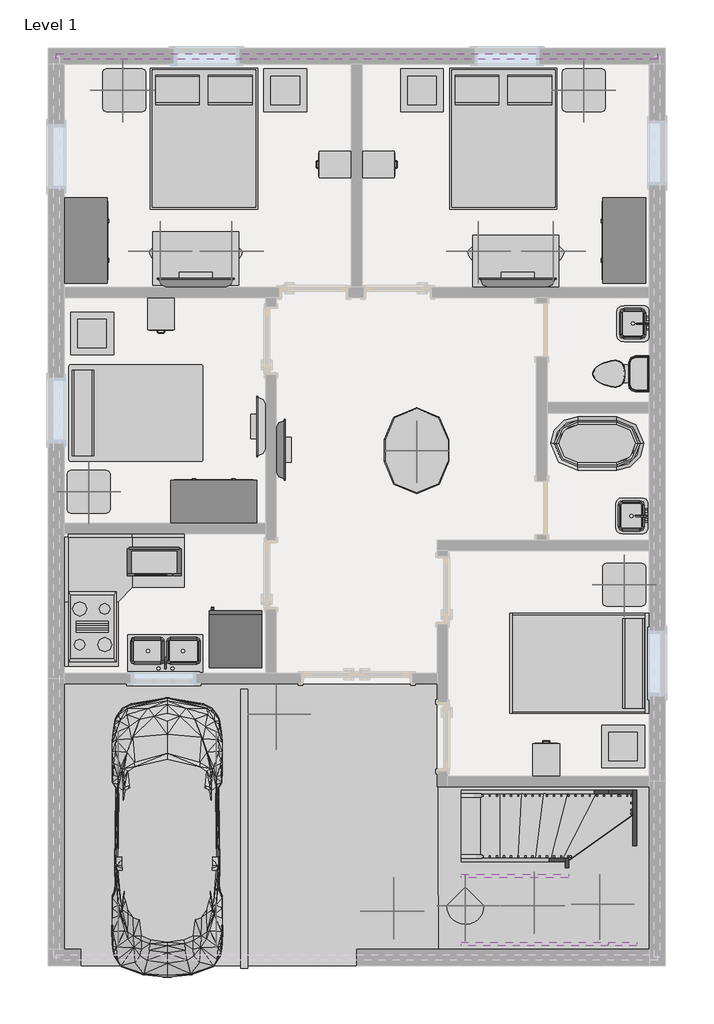
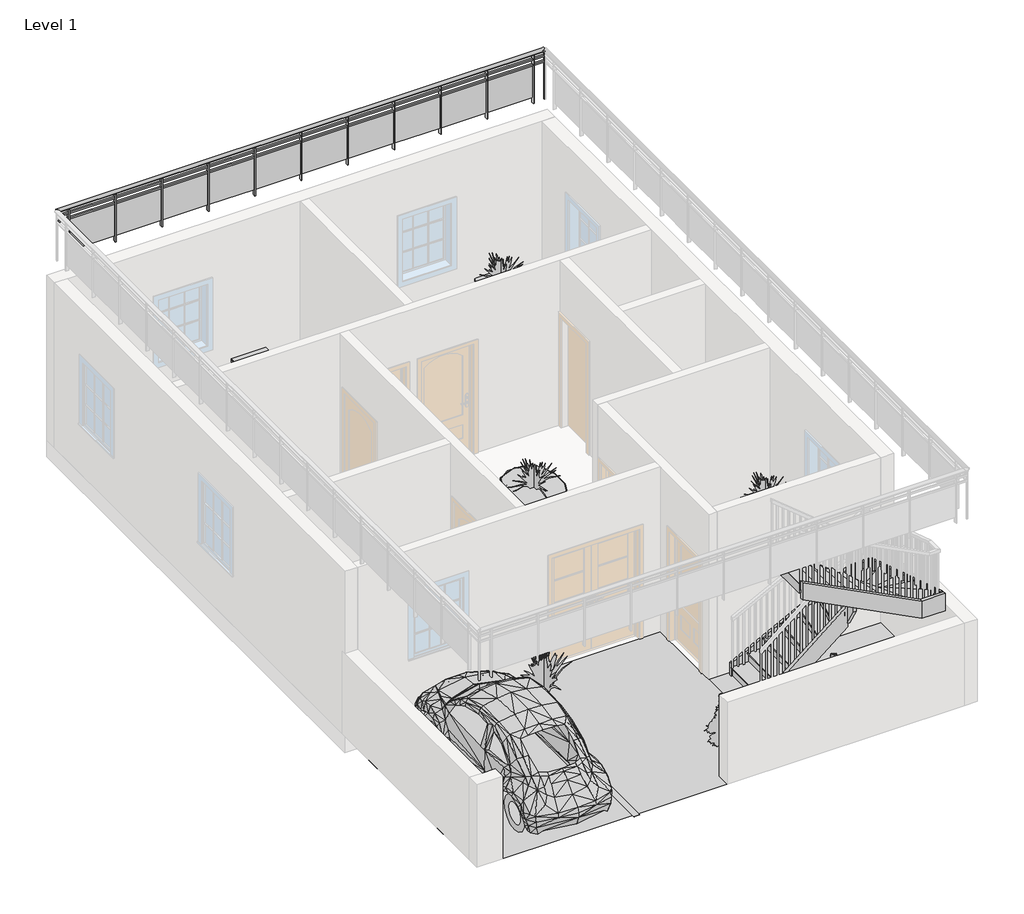
# One storey, part 4 of 4: 27 furniture elements, 14 geographic elements, 8 members, 7 flow terminals, 7 proxies, 1 railing, 1 stair flight.
"""IFC4 building model written with IfcOpenShell, lengths in millimetres."""

from ifc_helpers import new_model, si_unit, point, frame, origin, place, context, project, spatial, polyline, ellipse_curve, trimmed, outline, extrude, triangles, transform, mapped, element, save
from ifc_brep_helpers import plane_surface, extruded_surface, advanced_brep
from components import proxy_bb1e6e30, proxy_8a8d5ab2, parking_space_9_x_18_90_deg_c935943f, rpc_beetle_rpc_beetle_3ce7ba48, proxy_a13a33b2, flow_terminal_accce45a, flow_terminal_a53be723, flow_terminal_62a433f7, toilet_domestic_3d_toilet_domestic_3d_f7549cf7, toilet_domestic_3d_toilet_domestic_3d_183bbd19, flow_terminal_159a3241, furniture_1d2926bd, furniture_096e7f55, furniture_0253826f, furniture_bb55ed6b, furniture_9fa109b2, furniture_56245f3a, furniture_7a3aaa4f, furniture_b5c51a22, furniture_be1c6672, furniture_31d08a24, furniture_1bba2e14, furniture_005e41fd, rpc_plant_tropical_55f6ff97, rpc_plant_tropical_agave_1_5_93a2a214, rpc_plant_tropical_jungle_flame_3_9c4808c2, stair_flight_2bffc1af

model = new_model("IFC4")

# Units and contexts
model_context = context("Model", 3, world=origin())
ifc_project = project(units=[si_unit("LENGTHUNIT", "METRE", prefix="MILLI")], contexts=[model_context])

# Site, building, storey
site = spatial("IfcSite", under=ifc_project)
building = spatial("IfcBuilding", under=site)
storey = spatial("IfcBuildingStorey", under=building, Name="Level 1", Elevation=0.0)

# Proxies
placement = place(None, origin())
element("IfcBuildingElementProxy", 1, Name="Building Element Proxy", at=placement, inside=storey, context=model_context, shape_type="Tessellation", body=[
    triangles([(-12848.2506409, 4171.8645401, 0.0), (-7323.7506409, 4171.8645401, 0.0), (-7307.7033646, 171.3645946, 0.0), (-12848.2506409, 171.3645946, 0.0)], [[1, 4, 2], [3, 2, 4]], closed=False),
])
element("IfcBuildingElementProxy", 2, Name="Building Element Proxy", at=placement, inside=storey, context=model_context, shape_type="Tessellation", body=[
    triangles([(-7250.1225769, 171.3645946, 0.0), (-4085.2506409, 171.3645946, 0.0), (-4085.2506409, 2711.3647339, 0.0), (-7323.7506409, 2711.3647339, 0.0), (-7329.7188812, 171.3645946, 0.0)], [[4, 5, 1], [1, 2, 3], [1, 3, 4]], closed=False),
])
proxy_shape = proxy_bb1e6e30(model_context)
element("IfcBuildingElementProxy", 3, Name="Cook Top-4 Unit : 36\" x 20\"", ObjectType="Cook Top-4 Unit : 36\" x 20\"", at=placement, inside=storey, context=model_context, shape_type="MappedRepresentation", body=[
    mapped(proxy_shape, transform((-12225.9505662, 4984.6645941, 0.0), x_axis=(0.0, 1.0, 0.0), y_axis=(-1.0, 0.0, 0.0), z_axis=(0.0, 0.0, 1.0))),
])
proxy_2_shape = proxy_8a8d5ab2(model_context)
element("IfcBuildingElementProxy", 4, Name="Microwave : 30\" x 16\" x 18\"", ObjectType="Microwave : 30\" x 16\" x 18\"", at=placement, inside=storey, context=model_context, shape_type="MappedRepresentation", body=[
    mapped(proxy_2_shape, transform((-11843.5934435, 6264.8451, 0.0), x_axis=(1.0000000000000002, 0.0, 0.0), y_axis=(0.0, 1.0000000000000002, 0.0), z_axis=(0.0, 0.0, 1.0))),
])
parking_space_9_x_18_90_deg_shape = parking_space_9_x_18_90_deg_c935943f(model_context)
element("IfcBuildingElementProxy", 5, Name="Parking Space : 9' x 18' - 90 deg", ObjectType="Parking Space : 9' x 18' - 90 deg", at=placement, inside=storey, context=model_context, shape_type="MappedRepresentation", body=[
    mapped(parking_space_9_x_18_90_deg_shape, transform((-10066.9505662, 133.2645941, 0.0), x_axis=(-1.0000000000000004, 0.0, 0.0), y_axis=(0.0, -1.0000000000000004, 0.0), z_axis=(0.0, 0.0, 1.0))),
])
rpc_beetle_rpc_beetle_shape = rpc_beetle_rpc_beetle_3ce7ba48(model_context)
element("IfcBuildingElementProxy", 6, Name="RPC Beetle : RPC Beetle", ObjectType="RPC Beetle : RPC Beetle", at=placement, inside=storey, context=model_context, shape_type="MappedRepresentation", body=[
    mapped(rpc_beetle_rpc_beetle_shape, transform((-11159.1505662, 755.5645941, 0.0), x_axis=(1.0, 0.0, 0.0), y_axis=(0.0, 1.0, 0.0), z_axis=(0.0, 0.0, 1.0))),
])
proxy_3_shape = proxy_a13a33b2(model_context)
element("IfcBuildingElementProxy", 7, Name="Refrigerator : 30\" x 32\" RH", ObjectType="Refrigerator : 30\" x 32\" RH", at=placement, inside=storey, context=model_context, shape_type="MappedRepresentation", body=[
    mapped(proxy_3_shape, transform((-10186.0130662, 4792.9656227, 0.0), x_axis=(-1.0000000000000004, 0.0, 0.0), y_axis=(0.0, -1.0000000000000004, 0.0), z_axis=(0.0, 0.0, 1.0))),
])

# Flow terminals
flow_terminal_shape = flow_terminal_accce45a(model_context)
element("IfcFlowTerminal", 8, ObjectType="Floor Drain - Round : 5\" Strainer - 2\" Drain", at=placement, inside=storey, context=model_context, shape_type="MappedRepresentation", body=[
    mapped(flow_terminal_shape, transform((-4580.5505662, 7054.7645941, 0.0), x_axis=(1.0, 0.0, 0.0), y_axis=(0.0, 1.0, 0.0), z_axis=(0.0, 0.0, 1.0))),
])
element("IfcFlowTerminal", 9, ObjectType="Floor Drain - Round : 5\" Strainer - 2\" Drain", at=placement, inside=storey, context=model_context, shape_type="MappedRepresentation", body=[
    mapped(flow_terminal_shape, transform((-4529.7505662, 9455.0645941, 0.0), x_axis=(1.0, 0.0, 0.0), y_axis=(0.0, 1.0, 0.0), z_axis=(0.0, 0.0, 1.0))),
])
flow_terminal_2_shape = flow_terminal_a53be723(model_context)
element("IfcFlowTerminal", 10, ObjectType="Sink Kitchen-Double : 42\" x 21\"", at=placement, inside=storey, context=model_context, shape_type="MappedRepresentation", body=[
    mapped(flow_terminal_2_shape, transform((-11168.8613256, 4606.0099953, 0.0), x_axis=(-1.0000000000000004, 0.0, 0.0), y_axis=(0.0, -1.0000000000000004, 0.0), z_axis=(0.0, 0.0, 1.0))),
])
flow_terminal_3_shape = flow_terminal_62a433f7(model_context)
element("IfcFlowTerminal", 11, ObjectType="Sink Vanity-Square : 20\" x 18\"", at=placement, inside=storey, context=model_context, shape_type="MappedRepresentation", body=[
    mapped(flow_terminal_3_shape, transform((-4513.0459673, 6575.1538347, 0.0), x_axis=(0.0, -1.0000000000000004, 0.0), y_axis=(1.0000000000000004, 0.0, 0.0), z_axis=(0.0, 0.0, 1.0))),
])
element("IfcFlowTerminal", 12, ObjectType="Sink Vanity-Square : 20\" x 18\"", at=placement, inside=storey, context=model_context, shape_type="MappedRepresentation", body=[
    mapped(flow_terminal_3_shape, transform((-4493.9959673, 9305.6538347, 0.0), x_axis=(0.0, -1.0, 0.0), y_axis=(1.0, 0.0, 0.0), z_axis=(0.0, 0.0, 1.0))),
])
toilet_domestic_3d_toilet_domestic_3d_shape = toilet_domestic_3d_toilet_domestic_3d_f7549cf7(model_context)
toilet_domestic_3d_toilet_domestic_3d_2_shape = toilet_domestic_3d_toilet_domestic_3d_183bbd19(model_context)
element("IfcFlowTerminal", 13, ObjectType="Toilet-Domestic-3D : Toilet-Domestic-3D", at=placement, inside=storey, context=model_context, shape_type="MappedRepresentation", body=[
    mapped(toilet_domestic_3d_toilet_domestic_3d_shape, transform((-4808.5465935, 8578.7645941, 0.0), x_axis=(0.0, -1.0000000000000007, 0.0), y_axis=(1.0000000000000007, 0.0, 0.0), z_axis=(0.0, 0.0, 1.0))),
    mapped(toilet_domestic_3d_toilet_domestic_3d_2_shape, transform((-4808.5465935, 8578.7645941, 0.0), x_axis=(0.0, -1.0000000000000007, 0.0), y_axis=(1.0000000000000007, 0.0, 0.0), z_axis=(0.0, 0.0, 1.0))),
])
flow_terminal_4_shape = flow_terminal_159a3241(model_context)
element("IfcFlowTerminal", 14, ObjectType="Tub-Free Standing-3D : 30\" x 60\"", at=placement, inside=storey, context=model_context, shape_type="MappedRepresentation", body=[
    mapped(flow_terminal_4_shape, transform((-5050.4505662, 7588.1645941, 0.0), x_axis=(0.0, 1.0, 0.0), y_axis=(-1.0, 0.0, 0.0), z_axis=(0.0, 0.0, 1.0))),
])

# Furniture
furniture_shape = furniture_1d2926bd(model_context)
element("IfcFurniture", 15, ObjectType="Bed-Box : Queen 60\" x 79\"", at=placement, inside=storey, context=model_context, shape_type="MappedRepresentation", body=[
    mapped(furniture_shape, transform((-10977.6030252, 12153.2941023, 0.0), x_axis=(1.0000000000000004, 0.0, 0.0), y_axis=(0.0, 1.0000000000000004, 0.0), z_axis=(0.0, 0.0, 1.0))),
])
element("IfcFurniture", 16, ObjectType="Bed-Box : Queen 60\" x 79\"", at=placement, inside=storey, context=model_context, shape_type="MappedRepresentation", body=[
    mapped(furniture_shape, transform((-6723.1030252, 12153.2941023, 0.0), x_axis=(1.0, 0.0, 0.0), y_axis=(0.0, 1.0, 0.0), z_axis=(0.0, 0.0, 1.0))),
])
furniture_2_shape = furniture_096e7f55(model_context)
element("IfcFurniture", 17, ObjectType="Bed-Shaker : Double 56\" x 78\"", at=placement, inside=storey, context=model_context, shape_type="MappedRepresentation", body=[
    mapped(furniture_2_shape, transform((-4313.8505662, 4444.9145941, 0.0), x_axis=(0.0, -1.0000000000000004, 0.0), y_axis=(1.0000000000000004, 0.0, 0.0), z_axis=(0.0, 0.0, 1.0))),
])
furniture_3_shape = furniture_0253826f(model_context)
element("IfcFurniture", 18, ObjectType="Bed-Standard.0001 : Double 54\" x 75\"", at=placement, inside=storey, context=model_context, shape_type="MappedRepresentation", body=[
    mapped(furniture_3_shape, transform((-11649.2456481, 7748.4760696, 0.0), x_axis=(0.0, 1.0000000000000002, 0.0), y_axis=(-1.0000000000000002, 0.0, 0.0), z_axis=(0.0, 0.0, 1.0))),
])
furniture_4_shape = furniture_bb55ed6b(model_context)
element("IfcFurniture", 19, ObjectType="Cabinet-File 2 Drawer : 15\" x 18\"", at=placement, inside=storey, context=model_context, shape_type="MappedRepresentation", body=[
    mapped(furniture_4_shape, transform((-8629.416266, 11422.6681471, 0.0), x_axis=(0.0, -1.0000000000000004, 0.0), y_axis=(1.0000000000000004, 0.0, 0.0), z_axis=(0.0, 0.0, 1.0))),
])
element("IfcFurniture", 20, ObjectType="Cabinet-File 2 Drawer : 15\" x 18\"", at=placement, inside=storey, context=model_context, shape_type="MappedRepresentation", body=[
    mapped(furniture_4_shape, transform((-8304.0848663, 11678.4610412, 0.0), x_axis=(0.0, 1.0000000000000002, 0.0), y_axis=(-1.0000000000000002, 0.0, 0.0), z_axis=(0.0, 0.0, 1.0))),
])
element("IfcFurniture", 21, ObjectType="Cabinet-File 2 Drawer : 15\" x 18\"", at=placement, inside=storey, context=model_context, shape_type="MappedRepresentation", body=[
    mapped(furniture_4_shape, transform((-11120.1541191, 9571.7988943, 0.0), x_axis=(1.0, 0.0, 0.0), y_axis=(0.0, 1.0, 0.0), z_axis=(0.0, 0.0, 1.0))),
])
element("IfcFurniture", 22, ObjectType="Cabinet-File 2 Drawer : 15\" x 18\"", at=placement, inside=storey, context=model_context, shape_type="MappedRepresentation", body=[
    mapped(furniture_4_shape, transform((-5902.2470132, 2950.230294, 0.0), x_axis=(-1.0000000000000004, 0.0, 0.0), y_axis=(0.0, -1.0000000000000004, 0.0), z_axis=(0.0, 0.0, 1.0))),
])
furniture_5_shape = furniture_9fa109b2(model_context)
element("IfcFurniture", 23, ObjectType="Dresser : 48\" x 72\" x 24\"", at=placement, inside=storey, context=model_context, shape_type="MappedRepresentation", body=[
    mapped(furniture_5_shape, transform((-12678.0135203, 10740.257854, 0.0), x_axis=(0.0, 1.0000000000000002, 0.0), y_axis=(-1.0000000000000002, 0.0, 0.0), z_axis=(0.0, 0.0, 1.0))),
])
element("IfcFurniture", 24, ObjectType="Dresser : 48\" x 72\" x 24\"", at=placement, inside=storey, context=model_context, shape_type="MappedRepresentation", body=[
    mapped(furniture_5_shape, transform((-4306.2876121, 10201.8713343, 0.0), x_axis=(0.0, -1.0000000000000004, 0.0), y_axis=(1.0000000000000004, 0.0, 0.0), z_axis=(0.0, 0.0, 1.0))),
])
element("IfcFurniture", 25, ObjectType="Dresser : 48\" x 72\" x 24\"", at=placement, inside=storey, context=model_context, shape_type="MappedRepresentation", body=[
    mapped(furniture_5_shape, transform((-10767.943826, 6399.50164, 0.0), x_axis=(-1.0000000000000004, 0.0, 0.0), y_axis=(0.0, -1.0000000000000004, 0.0), z_axis=(0.0, 0.0, 1.0))),
])
furniture_6_shape = furniture_56245f3a(model_context)
element("IfcFurniture", 26, ObjectType="TV - Flat Screen : 32\"", at=placement, inside=storey, context=model_context, shape_type="MappedRepresentation", body=[
    mapped(furniture_6_shape, transform((-9820.6891898, 7825.52008, 0.0), x_axis=(0.0, -1.0000000000000004, 0.0), y_axis=(1.0000000000000004, 0.0, 0.0), z_axis=(0.0, 0.0, 1.0))),
])
element("IfcFurniture", 27, ObjectType="TV - Flat Screen : 32\"", at=placement, inside=storey, context=model_context, shape_type="MappedRepresentation", body=[
    mapped(furniture_6_shape, transform((-9551.2119425, 7503.2091083, 914.4), x_axis=(0.0, 1.0, 0.0), y_axis=(-1.0, 0.0, 0.0), z_axis=(0.0, 0.0, 1.0))),
])
furniture_7_shape = furniture_7a3aaa4f(model_context)
element("IfcFurniture", 28, ObjectType="TV - Flat Screen : 42\"", at=placement, inside=storey, context=model_context, shape_type="MappedRepresentation", body=[
    mapped(furniture_7_shape, transform((-10756.6950803, 9869.2032178, 1041.4), x_axis=(-1.0000000000000004, 0.0, 0.0), y_axis=(0.0, -1.0000000000000004, 0.0), z_axis=(0.0, 0.0, 1.0))),
])
element("IfcFurniture", 29, ObjectType="TV - Flat Screen : 42\"", at=placement, inside=storey, context=model_context, shape_type="MappedRepresentation", body=[
    mapped(furniture_7_shape, transform((-6184.6950803, 9869.2032178, 1041.4), x_axis=(-1.0000000000000002, 0.0, 0.0), y_axis=(0.0, -1.0000000000000002, 0.0), z_axis=(0.0, 0.0, 1.0))),
])
furniture_8_shape = furniture_b5c51a22(model_context)
element("IfcFurniture", 30, ObjectType="Table-Coffee : 24\" x 24\" x 24\"", at=placement, inside=storey, context=model_context, shape_type="MappedRepresentation", body=[
    mapped(furniture_8_shape, transform((-9501.0163328, 12509.4535163, 0.0), x_axis=(1.0, 0.0, 0.0), y_axis=(0.0, 1.0, 0.0), z_axis=(0.0, 0.0, 1.0))),
])
element("IfcFurniture", 31, ObjectType="Table-Coffee : 24\" x 24\" x 24\"", at=placement, inside=storey, context=model_context, shape_type="MappedRepresentation", body=[
    mapped(furniture_8_shape, transform((-7557.9163328, 12509.4535163, 0.0), x_axis=(1.0, 0.0, 0.0), y_axis=(0.0, 1.0, 0.0), z_axis=(0.0, 0.0, 1.0))),
])
element("IfcFurniture", 32, ObjectType="Table-Coffee : 24\" x 24\" x 24\"", at=placement, inside=storey, context=model_context, shape_type="MappedRepresentation", body=[
    mapped(furniture_8_shape, transform((-12244.2163328, 9055.0535163, 0.0), x_axis=(1.0, 0.0, 0.0), y_axis=(0.0, 1.0, 0.0), z_axis=(0.0, 0.0, 1.0))),
])
element("IfcFurniture", 33, ObjectType="Table-Coffee : 24\" x 24\" x 24\"", at=placement, inside=storey, context=model_context, shape_type="MappedRepresentation", body=[
    mapped(furniture_8_shape, transform((-4700.4163328, 3187.6535163, 0.0), x_axis=(1.0, 0.0, 0.0), y_axis=(0.0, 1.0, 0.0), z_axis=(0.0, 0.0, 1.0))),
])
furniture_9_shape = furniture_be1c6672(model_context)
element("IfcFurniture", 34, ObjectType="Table-Dining Oval : 36\" x 48\"", at=placement, inside=storey, context=model_context, shape_type="MappedRepresentation", body=[
    mapped(furniture_9_shape, transform((-7973.9489268, 7888.3842663, 0.0), x_axis=(0.0, 1.0000000000000002, 0.0), y_axis=(-1.0000000000000002, 0.0, 0.0), z_axis=(0.0, 0.0, 1.0))),
])
furniture_10_shape = furniture_31d08a24(model_context)
element("IfcFurniture", 35, ObjectType="Table-End : 24\" x 24\"", at=placement, inside=storey, context=model_context, shape_type="MappedRepresentation", body=[
    mapped(furniture_10_shape, transform((-12077.2841965, 12452.2645941, 0.0), x_axis=(1.0, 0.0, 0.0), y_axis=(0.0, 1.0, 0.0), z_axis=(0.0, 0.0, 1.0))),
])
element("IfcFurniture", 36, ObjectType="Table-End : 24\" x 24\"", at=placement, inside=storey, context=model_context, shape_type="MappedRepresentation", body=[
    mapped(furniture_10_shape, transform((-5549.4841965, 12452.2645941, 0.0), x_axis=(1.0, 0.0, 0.0), y_axis=(0.0, 1.0, 0.0), z_axis=(0.0, 0.0, 1.0))),
])
element("IfcFurniture", 37, ObjectType="Table-End : 24\" x 24\"", at=placement, inside=storey, context=model_context, shape_type="MappedRepresentation", body=[
    mapped(furniture_10_shape, transform((-12585.2841965, 6749.9645941, 0.0), x_axis=(1.0, 0.0, 0.0), y_axis=(0.0, 1.0, 0.0), z_axis=(0.0, 0.0, 1.0))),
])
element("IfcFurniture", 38, ObjectType="Table-End : 24\" x 24\"", at=placement, inside=storey, context=model_context, shape_type="MappedRepresentation", body=[
    mapped(furniture_10_shape, transform((-4977.9841965, 5429.1645941, 0.0), x_axis=(1.0, 0.0, 0.0), y_axis=(0.0, 1.0, 0.0), z_axis=(0.0, 0.0, 1.0))),
])
furniture_11_shape = furniture_1bba2e14(model_context)
element("IfcFurniture", 39, ObjectType="Table-Rectangular : 72\" x 30\"", at=placement, inside=storey, context=model_context, shape_type="MappedRepresentation", body=[
    mapped(furniture_11_shape, transform((-10752.7505662, 10217.0645941, 0.0), x_axis=(1.0, 0.0, 0.0), y_axis=(0.0, 1.0, 0.0), z_axis=(0.0, 0.0, 1.0))),
])
element("IfcFurniture", 40, ObjectType="Table-Rectangular : 72\" x 30\"", at=placement, inside=storey, context=model_context, shape_type="MappedRepresentation", body=[
    mapped(furniture_11_shape, transform((-6206.1505662, 10166.2645941, 0.0), x_axis=(1.0, 0.0, 0.0), y_axis=(0.0, 1.0, 0.0), z_axis=(0.0, 0.0, 1.0))),
])
furniture_12_shape = furniture_005e41fd(model_context)
element("IfcFurniture", 41, ObjectType="Work Station Cubicle : 96\" x 96\"", at=placement, inside=storey, context=model_context, shape_type="MappedRepresentation", body=[
    mapped(furniture_12_shape, transform((-12487.918814, 6800.4876018, 0.0), x_axis=(1.0, 0.0, 0.0), y_axis=(0.0, 1.0, 0.0), z_axis=(0.0, 0.0, 1.0))),
])

# Geographic elements
rpc_plant_tropical_shape = rpc_plant_tropical_55f6ff97(model_context)
element("IfcGeographicElement", 42, ObjectType="RPC Plant - Tropical", at=placement, inside=storey, context=model_context, shape_type="MappedRepresentation", body=[
    mapped(rpc_plant_tropical_shape, transform((-9609.7505662, 3740.0645941, 0.0), x_axis=(1.0, 0.0, 0.0), y_axis=(0.0, 1.0, 0.0), z_axis=(0.0, 0.0, 1.0))),
])
element("IfcGeographicElement", 43, ObjectType="RPC Plant - Tropical", at=placement, inside=storey, context=model_context, shape_type="MappedRepresentation", body=[
    mapped(rpc_plant_tropical_shape, transform((-6923.7005662, 1022.2645941, 0.0), x_axis=(1.0, 0.0, 0.0), y_axis=(0.0, 1.0, 0.0), z_axis=(0.0, 0.0, 1.0))),
])
element("IfcGeographicElement", 44, ObjectType="RPC Plant - Tropical", at=placement, inside=storey, context=model_context, shape_type="MappedRepresentation", body=[
    mapped(rpc_plant_tropical_shape, transform((-5011.6576808, 1041.3145941, 0.0), x_axis=(1.0, 0.0, 0.0), y_axis=(0.0, 1.0, 0.0), z_axis=(0.0, 0.0, 1.0))),
])
rpc_plant_tropical_agave_1_5_shape = rpc_plant_tropical_agave_1_5_93a2a214(model_context)
element("IfcGeographicElement", 45, ObjectType="RPC Plant - Tropical : Agave - 1.5'", at=placement, inside=storey, context=model_context, shape_type="MappedRepresentation", body=[
    mapped(rpc_plant_tropical_agave_1_5_shape, transform((-11794.1505662, 12604.6645941, 609.6), x_axis=(1.0, 0.0, 0.0), y_axis=(0.0, 1.0, 0.0), z_axis=(0.0, 0.0, 1.0))),
])
element("IfcGeographicElement", 46, ObjectType="RPC Plant - Tropical : Agave - 1.5'", at=placement, inside=storey, context=model_context, shape_type="MappedRepresentation", body=[
    mapped(rpc_plant_tropical_agave_1_5_shape, transform((-10244.7505662, 10318.6645941, 609.6), x_axis=(1.0, 0.0, 0.0), y_axis=(0.0, 1.0, 0.0), z_axis=(0.0, 0.0, 1.0))),
])
element("IfcGeographicElement", 47, ObjectType="RPC Plant - Tropical : Agave - 1.5'", at=placement, inside=storey, context=model_context, shape_type="MappedRepresentation", body=[
    mapped(rpc_plant_tropical_agave_1_5_shape, transform((-11260.7505662, 10318.6645941, 609.6), x_axis=(1.0, 0.0, 0.0), y_axis=(0.0, 1.0, 0.0), z_axis=(0.0, 0.0, 1.0))),
])
element("IfcGeographicElement", 48, ObjectType="RPC Plant - Tropical : Agave - 1.5'", at=placement, inside=storey, context=model_context, shape_type="MappedRepresentation", body=[
    mapped(rpc_plant_tropical_agave_1_5_shape, transform((-5240.9505662, 12604.6645941, 609.6), x_axis=(1.0, 0.0, 0.0), y_axis=(0.0, 1.0, 0.0), z_axis=(0.0, 0.0, 1.0))),
])
element("IfcGeographicElement", 49, ObjectType="RPC Plant - Tropical : Agave - 1.5'", at=placement, inside=storey, context=model_context, shape_type="MappedRepresentation", body=[
    mapped(rpc_plant_tropical_agave_1_5_shape, transform((-5672.7505662, 10318.6645941, 609.6), x_axis=(1.0, 0.0, 0.0), y_axis=(0.0, 1.0, 0.0), z_axis=(0.0, 0.0, 1.0))),
])
element("IfcGeographicElement", 50, ObjectType="RPC Plant - Tropical : Agave - 1.5'", at=placement, inside=storey, context=model_context, shape_type="MappedRepresentation", body=[
    mapped(rpc_plant_tropical_agave_1_5_shape, transform((-6739.5505662, 10318.6645941, 609.6), x_axis=(1.0, 0.0, 0.0), y_axis=(0.0, 1.0, 0.0), z_axis=(0.0, 0.0, 1.0))),
])
element("IfcGeographicElement", 51, ObjectType="RPC Plant - Tropical : Agave - 1.5'", at=placement, inside=storey, context=model_context, shape_type="MappedRepresentation", body=[
    mapped(rpc_plant_tropical_agave_1_5_shape, transform((-12276.7505662, 6902.3645941, 609.6), x_axis=(1.0, 0.0, 0.0), y_axis=(0.0, 1.0, 0.0), z_axis=(0.0, 0.0, 1.0))),
])
element("IfcGeographicElement", 52, ObjectType="RPC Plant - Tropical : Agave - 1.5'", at=placement, inside=storey, context=model_context, shape_type="MappedRepresentation", body=[
    mapped(rpc_plant_tropical_agave_1_5_shape, transform((-7615.8505662, 7486.5645941, 736.6), x_axis=(1.0, 0.0, 0.0), y_axis=(0.0, 1.0, 0.0), z_axis=(0.0, 0.0, 1.0))),
])
element("IfcGeographicElement", 53, ObjectType="RPC Plant - Tropical : Agave - 1.5'", at=placement, inside=storey, context=model_context, shape_type="MappedRepresentation", body=[
    mapped(rpc_plant_tropical_agave_1_5_shape, transform((-4669.4505662, 5581.5645941, 609.6), x_axis=(1.0, 0.0, 0.0), y_axis=(0.0, 1.0, 0.0), z_axis=(0.0, 0.0, 1.0))),
])
rpc_plant_tropical_jungle_flame_3_shape = rpc_plant_tropical_jungle_flame_3_9c4808c2(model_context)
element("IfcGeographicElement", 54, ObjectType="RPC Plant - Tropical : Jungle Flame - 3'", at=placement, inside=storey, context=model_context, shape_type="MappedRepresentation", body=[
    mapped(rpc_plant_tropical_jungle_flame_3_shape, transform((-5943.1015589, 1022.2645941, 0.0), x_axis=(1.0, 0.0, 0.0), y_axis=(0.0, 1.0, 0.0), z_axis=(0.0, 0.0, 1.0))),
])
element("IfcGeographicElement", 55, ObjectType="RPC Plant - Tropical : Jungle Flame - 3'", at=placement, inside=storey, context=model_context, shape_type="MappedRepresentation", body=[
    mapped(rpc_plant_tropical_jungle_flame_3_shape, transform((-7939.7005662, 946.0645941, 0.0), x_axis=(1.0, 0.0, 0.0), y_axis=(0.0, 1.0, 0.0), z_axis=(0.0, 0.0, 1.0))),
])

# Members
element("IfcMember", 56, ObjectType="Stringer - 2\" Width", at=placement, inside=storey, context=model_context, shape_type="SweptSolid", body=[
    extrude(outline(polyline([(229.639954, -6984.582258), (0.0, -6984.582258), (0.0, -6764.8199405), (962.500629, -4897.1650664), (1305.3956453, -4897.1650664), (229.639954, -6984.582258)])), frame((0.0, 2609.7645941, 0.0), z_axis=(0.0, 1.0, 0.0), x_axis=(0.0, 0.0, 1.0)), (0.0, 0.0, 1.0), 50.8),
])
element("IfcMember", 57, ObjectType="Stringer - 2\" Width", at=placement, inside=storey, context=model_context, shape_type="SweptSolid", body=[
    extrude(outline(polyline([(-4897.1650664, 2609.7645941), (-4897.1650664, 2660.5645941), (-4542.4505662, 2660.5645941), (-4542.4505662, 2609.7645941), (-4897.1650664, 2609.7645941)])), frame((0.0, 0.0, 962.500629), z_axis=(0.0, 0.0, 1.0), x_axis=(1.0, 0.0, 0.0)), (0.0, 0.0, 1.0), 342.8950162),
])
element("IfcMember", 58, ObjectType="Stringer - 2\" Width", at=placement, inside=storey, context=model_context, shape_type="SweptSolid", body=[
    extrude(outline(polyline([(2660.5645941, 1289.0952212), (2660.5645941, 1000.5956453), (2491.0421112, 1000.5956453), (501.5645941, 1638.9682298), (501.5645941, 1969.9972697), (538.5447114, 1969.9972697), (2660.5645941, 1289.0952212)])), frame((-4542.4505662, 0.0, 0.0), z_axis=(1.0, 0.0, 0.0), x_axis=(0.0, 1.0, 0.0)), (0.0, 0.0, 1.0), 50.8),
])
element("IfcMember", 59, ObjectType="Stringer - 2\" Width", at=placement, inside=storey, context=model_context, shape_type="SweptSolid", body=[
    extrude(outline(polyline([(-4491.6505662, 501.5645941), (-4491.6505662, 450.7645941), (-4897.1650664, 450.7645941), (-4897.1650664, 501.5645941), (-4491.6505662, 501.5645941)])), frame((0.0, 0.0, 1649.8904473), z_axis=(0.0, 0.0, 1.0), x_axis=(1.0, 0.0, 0.0)), (0.0, 0.0, 1.0), 320.1068224),
])
element("IfcMember", 60, ObjectType="Stringer - 2\" Width", at=placement, inside=storey, context=model_context, shape_type="SweptSolid", body=[
    extrude(outline(polyline([(1649.8904473, -4897.1650664), (1969.9972697, -4897.1650664), (3045.7529609, -6984.582258), (2725.6461385, -6984.582258), (1649.8904473, -4897.1650664)])), frame((0.0, 450.7645941, 0.0), z_axis=(0.0, 1.0, 0.0), x_axis=(0.0, 0.0, 1.0)), (0.0, 0.0, 1.0), 50.8),
])
element("IfcMember", 61, ObjectType="Stringer - 2\" Width", at=placement, inside=storey, context=model_context, shape_type="SweptSolid", body=[
    extrude(outline(polyline([(176.1764461, -6984.582258), (0.0, -6984.582258), (0.0, -6718.3206135), (987.1410923, -5507.6505662), (1380.418648, -5507.6505662), (176.1764461, -6984.582258)])), frame((0.0, 1644.5645941, 0.0), z_axis=(0.0, 1.0, 0.0), x_axis=(0.0, 0.0, 1.0)), (0.0, 0.0, 1.0), 50.8),
])
element("IfcMember", 62, ObjectType="Stringer - 2\" Width", at=placement, inside=storey, context=model_context, shape_type="SweptSolid", body=[
    extrude(outline(polyline([(1695.3645941, 1573.2682978), (1695.3645941, 1028.5617647), (1661.1223768, 1028.5617647), (1466.7645941, 1360.465107), (1466.7645941, 1926.1409689), (1488.7274767, 1926.1409689), (1695.3645941, 1573.2682978)])), frame((-5507.6505662, 0.0, 0.0), z_axis=(1.0, 0.0, 0.0), x_axis=(0.0, 1.0, 0.0)), (0.0, 0.0, 1.0), 50.8),
])
element("IfcMember", 63, ObjectType="Stringer - 2\" Width", at=placement, inside=storey, context=model_context, shape_type="SweptSolid", body=[
    extrude(outline(polyline([(1532.8634131, -5456.8505662), (1926.1409689, -5456.8505662), (3171.8038432, -6984.582258), (2778.5262875, -6984.582258), (1532.8634131, -5456.8505662)])), frame((0.0, 1415.9645941, 0.0), z_axis=(0.0, 1.0, 0.0), x_axis=(0.0, 0.0, 1.0)), (0.0, 0.0, 1.0), 50.8),
])

# Railing
element("IfcRailing", 64, ObjectType="Glass Panel - Bottom Fill", at=placement, inside=storey, context=model_context, shape_type="SolidModel", body=[
    advanced_brep(
    [(-12733.9505662, 13125.3645941, 4267.2), (-12733.9505662, 13049.1645941, 4267.2), (-4199.5505662, 13125.3645941, 4267.2), (-4199.5505662, 13049.1645941, 4267.2)],
    [
        (0, 1, ellipse_curve(frame((-12733.9505662, 13087.2645941, 4267.2), z_axis=(-1.0, 0.0, 0.0), x_axis=(0.0, -1.0, 0.0)), 38.1, 28.575)),
        (1, 0, ellipse_curve(frame((-12733.9505662, 13087.2645941, 4267.2), z_axis=(-1.0, 0.0, 0.0), x_axis=(0.0, -1.0, 0.0)), 38.1, 28.575)),
        (2, 3, ellipse_curve(frame((-4199.5505662, 13087.2645941, 4267.2), z_axis=(1.0, 0.0, 0.0), x_axis=(0.0, -1.0, 0.0)), 38.1, 28.575)),
        (3, 2, ellipse_curve(frame((-4199.5505662, 13087.2645941, 4267.2), z_axis=(1.0, 0.0, 0.0), x_axis=(0.0, -1.0, 0.0)), 38.1, 28.575)),
        (0, 2),
        (3, 1),
    ],
    [
        plane_surface(frame((-12733.9505662, 13087.2645941, 4267.2), z_axis=(-1.0, 0.0, 0.0), x_axis=(0.0, 1.0, 0.0))),
        plane_surface(frame((-4199.5505662, 13087.2645941, 4267.2), z_axis=(1.0, 0.0, 0.0), x_axis=(0.0, 1.0, 0.0))),
        extruded_surface(trimmed(ellipse_curve(frame((-4199.5505662, 13087.2645941, 4267.2), z_axis=(-1.0, 0.0, 0.0), x_axis=(0.0, -1.0, 0.0)), 38.1, 28.575), [point((-4199.5505662, 13125.3645941, 4267.2))], [point((-4199.5505662, 13049.1645941, 4267.2))], True, "CARTESIAN"), (-8534.4, 0.0, 0.0), 8534.4),
        extruded_surface(trimmed(ellipse_curve(frame((-4199.5505662, 13087.2645941, 4267.2), z_axis=(-1.0, 0.0, 0.0), x_axis=(0.0, -1.0, 0.0)), 38.1, 28.575), [point((-4199.5505662, 13049.1645941, 4267.2))], [point((-4199.5505662, 13125.3645941, 4267.2))], True, "CARTESIAN"), (-8534.4, 0.0, 0.0), 8534.4),
    ],
    [
        (0, [[1, 2]]),
        (1, [[3, 4]]),
        (2, [[-1, 5, -4, 6]]),
        (3, [[-2, -6, -3, -5]]),
    ],
),
    extrude(outline(polyline([(-12733.9505662, 13074.5645941), (-12733.9505662, 13099.9645941), (-4199.5505662, 13099.9645941), (-4199.5505662, 13074.5645941), (-12733.9505662, 13074.5645941)])), frame((0.0, 0.0, 4152.9), z_axis=(0.0, 0.0, 1.0), x_axis=(1.0, 0.0, 0.0)), (0.0, 0.0, 1.0), 25.4),
    extrude(outline(polyline([(-12733.9505662, 13074.5645941), (-12733.9505662, 13099.9645941), (-4199.5505662, 13099.9645941), (-4199.5505662, 13074.5645941), (-12733.9505662, 13074.5645941)])), frame((0.0, 0.0, 4051.3), z_axis=(0.0, 0.0, 1.0), x_axis=(1.0, 0.0, 0.0)), (0.0, 0.0, 1.0), 25.4),
    extrude(outline(polyline([(-4409.1005662, 13061.8645941), (-4409.1005662, 13112.6645941), (-4396.4005662, 13112.6645941), (-4396.4005662, 13061.8645941), (-4409.1005662, 13061.8645941)])), frame((0.0, 0.0, 3352.8), z_axis=(0.0, 0.0, 1.0), x_axis=(1.0, 0.0, 0.0)), (0.0, 0.0, 1.0), 885.6788223),
    extrude(outline(polyline([(-5215.5505662, 13093.7997511), (-4402.7505662, 13093.7997511), (-4402.7505662, 13087.4497511), (-5215.5505662, 13087.4497511), (-5215.5505662, 13093.7997511)])), frame((0.0, 0.0, 3454.4), z_axis=(0.0, 0.0, 1.0), x_axis=(1.0, 0.0, 0.0)), (0.0, 0.0, 1.0), 596.9),
    extrude(outline(polyline([(-5221.9005662, 13061.8645941), (-5221.9005662, 13112.6645941), (-5209.2005662, 13112.6645941), (-5209.2005662, 13061.8645941), (-5221.9005662, 13061.8645941)])), frame((0.0, 0.0, 3352.8), z_axis=(0.0, 0.0, 1.0), x_axis=(1.0, 0.0, 0.0)), (0.0, 0.0, 1.0), 885.6788223),
    extrude(outline(polyline([(-6028.3505662, 13093.7997511), (-5215.5505662, 13093.7997511), (-5215.5505662, 13087.4497511), (-6028.3505662, 13087.4497511), (-6028.3505662, 13093.7997511)])), frame((0.0, 0.0, 3454.4), z_axis=(0.0, 0.0, 1.0), x_axis=(1.0, 0.0, 0.0)), (0.0, 0.0, 1.0), 596.9),
    extrude(outline(polyline([(-6034.7005662, 13061.8645941), (-6034.7005662, 13112.6645941), (-6022.0005662, 13112.6645941), (-6022.0005662, 13061.8645941), (-6034.7005662, 13061.8645941)])), frame((0.0, 0.0, 3352.8), z_axis=(0.0, 0.0, 1.0), x_axis=(1.0, 0.0, 0.0)), (0.0, 0.0, 1.0), 885.6788223),
    extrude(outline(polyline([(-6841.1505662, 13093.7997511), (-6028.3505662, 13093.7997511), (-6028.3505662, 13087.4497511), (-6841.1505662, 13087.4497511), (-6841.1505662, 13093.7997511)])), frame((0.0, 0.0, 3454.4), z_axis=(0.0, 0.0, 1.0), x_axis=(1.0, 0.0, 0.0)), (0.0, 0.0, 1.0), 596.9),
    extrude(outline(polyline([(-6847.5005662, 13061.8645941), (-6847.5005662, 13112.6645941), (-6834.8005662, 13112.6645941), (-6834.8005662, 13061.8645941), (-6847.5005662, 13061.8645941)])), frame((0.0, 0.0, 3352.8), z_axis=(0.0, 0.0, 1.0), x_axis=(1.0, 0.0, 0.0)), (0.0, 0.0, 1.0), 885.6788223),
    extrude(outline(polyline([(-7653.9505662, 13093.7997511), (-6841.1505662, 13093.7997511), (-6841.1505662, 13087.4497511), (-7653.9505662, 13087.4497511), (-7653.9505662, 13093.7997511)])), frame((0.0, 0.0, 3454.4), z_axis=(0.0, 0.0, 1.0), x_axis=(1.0, 0.0, 0.0)), (0.0, 0.0, 1.0), 596.9),
    extrude(outline(polyline([(-7660.3005662, 13061.8645941), (-7660.3005662, 13112.6645941), (-7647.6005662, 13112.6645941), (-7647.6005662, 13061.8645941), (-7660.3005662, 13061.8645941)])), frame((0.0, 0.0, 3352.8), z_axis=(0.0, 0.0, 1.0), x_axis=(1.0, 0.0, 0.0)), (0.0, 0.0, 1.0), 885.6788223),
    extrude(outline(polyline([(-8466.7505662, 13093.7997511), (-7653.9505662, 13093.7997511), (-7653.9505662, 13087.4497511), (-8466.7505662, 13087.4497511), (-8466.7505662, 13093.7997511)])), frame((0.0, 0.0, 3454.4), z_axis=(0.0, 0.0, 1.0), x_axis=(1.0, 0.0, 0.0)), (0.0, 0.0, 1.0), 596.9),
    extrude(outline(polyline([(-8473.1005662, 13061.8645941), (-8473.1005662, 13112.6645941), (-8460.4005662, 13112.6645941), (-8460.4005662, 13061.8645941), (-8473.1005662, 13061.8645941)])), frame((0.0, 0.0, 3352.8), z_axis=(0.0, 0.0, 1.0), x_axis=(1.0, 0.0, 0.0)), (0.0, 0.0, 1.0), 885.6788223),
    extrude(outline(polyline([(-9279.5505662, 13093.7997511), (-8466.7505662, 13093.7997511), (-8466.7505662, 13087.4497511), (-9279.5505662, 13087.4497511), (-9279.5505662, 13093.7997511)])), frame((0.0, 0.0, 3454.4), z_axis=(0.0, 0.0, 1.0), x_axis=(1.0, 0.0, 0.0)), (0.0, 0.0, 1.0), 596.9),
    extrude(outline(polyline([(-9285.9005662, 13061.8645941), (-9285.9005662, 13112.6645941), (-9273.2005662, 13112.6645941), (-9273.2005662, 13061.8645941), (-9285.9005662, 13061.8645941)])), frame((0.0, 0.0, 3352.8), z_axis=(0.0, 0.0, 1.0), x_axis=(1.0, 0.0, 0.0)), (0.0, 0.0, 1.0), 885.6788223),
    extrude(outline(polyline([(-10092.3505662, 13093.7997511), (-9279.5505662, 13093.7997511), (-9279.5505662, 13087.4497511), (-10092.3505662, 13087.4497511), (-10092.3505662, 13093.7997511)])), frame((0.0, 0.0, 3454.4), z_axis=(0.0, 0.0, 1.0), x_axis=(1.0, 0.0, 0.0)), (0.0, 0.0, 1.0), 596.9),
    extrude(outline(polyline([(-10098.7005662, 13061.8645941), (-10098.7005662, 13112.6645941), (-10086.0005662, 13112.6645941), (-10086.0005662, 13061.8645941), (-10098.7005662, 13061.8645941)])), frame((0.0, 0.0, 3352.8), z_axis=(0.0, 0.0, 1.0), x_axis=(1.0, 0.0, 0.0)), (0.0, 0.0, 1.0), 885.6788223),
    extrude(outline(polyline([(-10905.1505662, 13093.7997511), (-10092.3505662, 13093.7997511), (-10092.3505662, 13087.4497511), (-10905.1505662, 13087.4497511), (-10905.1505662, 13093.7997511)])), frame((0.0, 0.0, 3454.4), z_axis=(0.0, 0.0, 1.0), x_axis=(1.0, 0.0, 0.0)), (0.0, 0.0, 1.0), 596.9),
    extrude(outline(polyline([(-10911.5005662, 13061.8645941), (-10911.5005662, 13112.6645941), (-10898.8005662, 13112.6645941), (-10898.8005662, 13061.8645941), (-10911.5005662, 13061.8645941)])), frame((0.0, 0.0, 3352.8), z_axis=(0.0, 0.0, 1.0), x_axis=(1.0, 0.0, 0.0)), (0.0, 0.0, 1.0), 885.6788223),
    extrude(outline(polyline([(-11717.9505662, 13093.7997511), (-10905.1505662, 13093.7997511), (-10905.1505662, 13087.4497511), (-11717.9505662, 13087.4497511), (-11717.9505662, 13093.7997511)])), frame((0.0, 0.0, 3454.4), z_axis=(0.0, 0.0, 1.0), x_axis=(1.0, 0.0, 0.0)), (0.0, 0.0, 1.0), 596.9),
    extrude(outline(polyline([(-11724.3005662, 13061.8645941), (-11724.3005662, 13112.6645941), (-11711.6005662, 13112.6645941), (-11711.6005662, 13061.8645941), (-11724.3005662, 13061.8645941)])), frame((0.0, 0.0, 3352.8), z_axis=(0.0, 0.0, 1.0), x_axis=(1.0, 0.0, 0.0)), (0.0, 0.0, 1.0), 885.6788223),
    extrude(outline(polyline([(-12530.7505662, 13093.7997511), (-11717.9505662, 13093.7997511), (-11717.9505662, 13087.4497511), (-12530.7505662, 13087.4497511), (-12530.7505662, 13093.7997511)])), frame((0.0, 0.0, 3454.4), z_axis=(0.0, 0.0, 1.0), x_axis=(1.0, 0.0, 0.0)), (0.0, 0.0, 1.0), 596.9),
    extrude(outline(polyline([(-12537.1005662, 13061.8645941), (-12537.1005662, 13112.6645941), (-12524.4005662, 13112.6645941), (-12524.4005662, 13061.8645941), (-12537.1005662, 13061.8645941)])), frame((0.0, 0.0, 3352.8), z_axis=(0.0, 0.0, 1.0), x_axis=(1.0, 0.0, 0.0)), (0.0, 0.0, 1.0), 885.6788223),
    extrude(outline(polyline([(-4212.2505662, 13077.7395941), (-4212.2505662, 13096.7895941), (-4193.2005662, 13096.7895941), (-4193.2005662, 13077.7395941), (-4212.2505662, 13077.7395941)])), frame((0.0, 0.0, 3352.8), z_axis=(0.0, 0.0, 1.0), x_axis=(1.0, 0.0, 0.0)), (0.0, 0.0, 1.0), 885.6788223),
    extrude(outline(polyline([(-12740.3005662, 13077.7395941), (-12740.3005662, 13096.7895941), (-12721.2505662, 13096.7895941), (-12721.2505662, 13077.7395941), (-12740.3005662, 13077.7395941)])), frame((0.0, 0.0, 3352.8), z_axis=(0.0, 0.0, 1.0), x_axis=(1.0, 0.0, 0.0)), (0.0, 0.0, 1.0), 885.6788223),
])

# Stair flight
stair_flight_shape = stair_flight_2bffc1af(model_context)
element("IfcStairFlight", 65, ObjectType="2\" Tread 1\" Nosing 1/4\" Riser", at=placement, inside=storey, context=model_context, shape_type="MappedRepresentation", body=[
    mapped(stair_flight_shape, transform((0.0, 0.0, 0.0), x_axis=(1.0, 0.0, 0.0), y_axis=(0.0, 1.0, 0.0), z_axis=(0.0, 0.0, 1.0))),
])

save(model, "model.ifc")

# Revit data of these elements
# Type "Cook Top-4 Unit : 36\" x 20\""
#   Assembly Code = "E1090400"
#   Depth = 2' - 0"
#   Width = 3' - 0"
#   Burner Material = Steel, Chrome Plated
#   Cooktop Material = Steel, Polished
#   Default Elevation = 0
# Type "Microwave : 30\" x 16\" x 18\""
#   Assembly Code = "E1090400"
#   Depth = 1' - 4"
#   Height = 1' - 6"
#   Width = 2' - 6"
#   Microwave Material = Laminate - Ivory, Glossy
#   Default Elevation = 0
# Type "Parking Space : 9' x 18' - 90 deg"
#   Angle = 90.00°
#   Parking Length = 18' - 0"
#   Parking Width = 9' - 0"
#   pl = 13' - 0"
#   pw = 7' - 0"
# Type "RPC Beetle : RPC Beetle"
#   built-in parameter 1005195 = "RPC-16-0U6E-L4EG-ENH1-J3KF-SVEL-0TX4-C0"
#   Height = 0
# Type "Refrigerator : 30\" x 32\" RH"
#   Label = "REF."
#   Assembly Code = "E1090400"
#   Depth = 2' - 7 3/4"
#   Handle = 2' - 3"
#   Height = 5' - 10"
#   Rear Clearance = 0' - 2"
#   Top Door Height = 1' - 8"
#   Width = 2' - 5 3/8"
#   Material = Steel, Chrome Plated
#   Default Elevation = 0
# Type "Floor Drain - Round : 5\" Strainer - 2\" Drain"
#   WFU = 2
#   Strainer Height = 0' - 3 1/4"
#   Strainer Radius = 0' - 2 1/2"
#   Strainer Diameter = 0' - 5"
#   Radius 6 = 0' - 0 5/8"
#   Radius 5 = 0' - 1 1/4"
#   Radius 4 = 0' - 1 7/8"
#   Radius 2 = 0' - 3.04167"
#   Radius 1 = 0' - 2.02083"
#   Radius 3 = 0' - 2 1/32"
#   Pipe Radius = 1"
#   Pipe Diameter = 2"
#   Height 2 = 0' - 0.725"
#   Height 1 = 0' - 1 13/16"
#   Body Radius = 0' - 4 1/16"
#   Body Height = 0' - 3 5/8"
#   Body Diameter = 0' - 8 1/8"
#   Drain Material = none
#   HWFU = 0
#   Default Elevation = 0
#   CWFU = 0
# Type "Sink Kitchen-Double : 42\" x 21\""
#   Assembly Code = "D2010410"
#   Counter Height = 3' - 0"
#   Depth = 1' - 9"
#   Width = 3' - 6"
#   Faucet Material = Steel, Polished
#   Sink Material = Steel, Polished
#   Default Elevation = 0
# Type "Sink Vanity-Square : 20\" x 18\""
#   Assembly Code = "D2010400"
#   Counter Height = 2' - 7"
#   Depth = 1' - 6"
#   Width = 1' - 8"
#   Basin Material = Porcelain, Linen
#   Faucet Material = Steel, Polished
#   Default Elevation = 0
# Type "Toilet-Domestic-3D : Toilet-Domestic-3D"
#   Assembly Code = "D2010110"
#   Toilet - Bowl/Basin Material = Porcelain, Linen
#   Toilet - Seat Material = Laminate, Linen, Matte
#   Default Elevation = 0
# Type "Tub-Free Standing-3D : 30\" x 60\""
#   Assembly Code = "D2010110"
#   Height = 1' - 6"
#   Length = 4' - 4"
#   Width = 2' - 6"
#   Tub Material = Porcelain, Ivory
#   Default Elevation = 0
# Type "Bed-Box : Queen 60\" x 79\""
#   Assembly Code = "E2020200"
#   Length = 6' - 7"
#   Width = 5' - 0"
#   Frame Material = Birch
#   Mattress Material = Softwood, Lumber
#   Default Elevation = 0
# Type "Bed-Shaker : Double 56\" x 78\""
#   Assembly Code = "E2020200"
#   Length = 6' - 6"
#   Width = 4' - 8"
#   Frame Material = Birch
#   Mattress Material = Plywood, Sheathing
#   Default Elevation = 0
# Type "Bed-Standard.0001 : Double 54\" x 75\""
#   Assembly Code = "E2020200"
#   Length = 6' - 3"
#   Width = 4' - 6"
#   Leg Material = Steel, Chrome Plated
#   Mattress Material = Linen, White
#   Default Elevation = 0
# Type "Cabinet-File 2 Drawer : 15\" x 18\""
#   Assembly Code = "E2020200"
#   Depth = 1' - 6"
#   Height = 2' - 5"
#   Width = 1' - 3"
#   Cabinet Material = Steel, Paint Finish, Ivory, Glossy
#   Handle Material = Steel, Chrome Plated
#   Default Elevation = 0
# Type "Dresser : 48\" x 72\" x 24\""
#   Assembly Code = "E2020200"
#   Depth = 2' - 0"
#   Height = 6' - 0"
#   Width = 4' - 0"
#   Dresser Material = Wood - Teak
#   Drawer Material = Wood - Teak
#   Knob Material = Cherry
#   Default Elevation = 0
# Type "TV - Flat Screen : 32\""
#   SinAng = 0' - 0.0193"
#   L = 2' - 3.79372"
#   H = 1' - 3.6354"
#   Thickness = 0' - 4.33071"
#   Diagonal = 2' - 7.88976"
#   CosAng = 0' - 0.03431"
#   Stand [instance default] = yes
#   Default Elevation = 0
# Type "TV - Flat Screen : 42\""
#   SinAng = 0' - 0.0193"
#   L = 3' - 0.71517"
#   H = 1' - 8.65418"
#   Thickness = 0' - 4.33071"
#   Diagonal = 3' - 6.12598"
#   CosAng = 0' - 0.03431"
#   Stand [instance default] = yes
#   Default Elevation = 0
# Type "Table-Coffee : 24\" x 24\" x 24\""
#   Assembly Code = "E2020200"
#   Height = 2' - 0"
#   Length = 2' - 0"
#   Width = 2' - 0"
#   Top Material = none
#   Frame Material = none
#   Default Elevation = 0
# Type "Table-Dining Oval : 36\" x 48\""
#   Assembly Code = "E2020200"
#   Length = 4' - 0"
#   Width = 3' - 0"
#   Base Material = Steel, Chrome Plated
#   Top Material = Glass - Clear, Grey
#   Default Elevation = 0
#   Description = (empty or 0)
# Type "Table-End : 24\" x 24\""
#   Assembly Code = "E2020200"
#   Height = 2' - 0"
#   Length = 2' - 0"
#   Width = 2' - 0"
#   Base Material = Birch
#   Top Material = Laminate, Ivory, Matte
#   Default Elevation = 0
# Type "Table-Rectangular : 72\" x 30\""
#   Assembly Code = "E2020200"
#   Height = 2' - 0"
#   Length = 4' - 0"
#   Width = 2' - 6"
#   Base Material = Birch
#   Top Material = Birch
#   Default Elevation = 0
# Type "Work Station Cubicle : 96\" x 96\""
#   Assembly Code = "E2020"
#   Desktop Height = 2' - 6"
#   Desktop1 Width = 2' - 4"
#   Desktop2 Width = 2' - 4"
#   Panel Height = 2' - 8"
#   Panel1 Length = 3' - 0"
#   Panel2 Length = 2' - 5"
#   Cube Panel Material = Textile - Light Gray
#   Work Top Material = Laminate, Ivory, Matte
#   Default Elevation = 0
# Type "RPC Plant - Tropical"
#   built-in parameter 1005198 = "{2, 15},{39, RPC-16-FWM5-GM7X-C67P-4000-ST1L-LVER-AU},{1, 0},{1, 0},{2, 13},{1, 8},{5, Color},{1, 0},{1, 0},{3, 0.8},{3, 0.8},{3, 0.8},{1, 8},{7, BBoxMin},{1, 0},{1, 0},{1, 0},{1, 0},{1, 0},{1, 8},{7, BBoxMax},{1, 0},{1, 0},{1, 0},{1, 0},{1, 0},{2, 11},{9, RPCTypeId},{1, 0},{1, 0},{39, RPC-16-FWM5-GM7X-C67P-4000-ST1L-LVER-AU},{1, 6},{14, RPCPlantHeight},{1, 0},{1, 0},{1, 3},{2, 11},{7, keyword},{1, 0},{1, 0},{35, :RPCs:Shrubs [General]:Geometry:RPC},{2, 11},{8, category},{1, 0},{1, 0},{16, Shrubs [General]},{2, 11},{12, LocalizedUID},{1, 0},{1, 0},{10, Crane Lily},{2, 14},{6, Height},{1, 0},{1, 0},{1, 3},{1, 2},{16, Cast Reflections},{1, 0},{1, 0},{1, 0},{1, 2},{12, Cast Shadows},{1, 0},{1, 0},{1, 1},{1, 2},{9, Lock View},{1, 0},{1, 0},{1, 0},{1, 4},{5, ViewC},{1, 0},{1, 0},{1, 0},{21, assetlibrary_base.fbx},{1, 5},"
#   built-in parameter 1005195 = "RPC-16-FWM5-GM7X-C67P-4000-ST1L-LVER-AU"
#   Assembly Code = "G2050500"
#   Height = 3' - 0"
#   Default Elevation = 0
# Type "RPC Plant - Tropical : Agave - 1.5'"
#   built-in parameter 1005198 = "{2, 15},{39, RPC-16-G1GJ-63FX-7K5P-N000-ST1L-LVER-AU},{1, 0},{1, 0},{2, 13},{1, 8},{5, Color},{1, 0},{1, 0},{3, 0.8},{3, 0.8},{3, 0.8},{1, 8},{7, BBoxMin},{1, 0},{1, 0},{1, 0},{1, 0},{1, 0},{1, 8},{7, BBoxMax},{1, 0},{1, 0},{1, 0},{1, 0},{1, 0},{2, 11},{9, RPCTypeId},{1, 0},{1, 0},{39, RPC-16-G1GJ-63FX-7K5P-N000-ST1L-LVER-AU},{1, 6},{14, RPCPlantHeight},{1, 0},{1, 0},{3, 1.5},{2, 11},{7, keyword},{1, 0},{1, 0},{35, :RPCs:Plants [General]:Geometry:RPC},{2, 11},{8, category},{1, 0},{1, 0},{16, Plants [General]},{2, 11},{12, LocalizedUID},{1, 0},{1, 0},{5, Agave},{2, 14},{6, Height},{1, 0},{1, 0},{3, 1.5},{1, 2},{16, Cast Reflections},{1, 0},{1, 0},{1, 0},{1, 2},{12, Cast Shadows},{1, 0},{1, 0},{1, 1},{1, 2},{9, Lock View},{1, 0},{1, 0},{1, 0},{1, 4},{5, ViewC},{1, 0},{1, 0},{1, 0},{21, assetlibrary_base.fbx},{1, 5},"
#   built-in parameter 1005195 = "RPC-16-G1GJ-63FX-7K5P-N000-ST1L-LVER-AU"
#   Type Comments = "Agave"
#   Assembly Code = "G2050500"
#   Height = 1' - 6"
#   Default Elevation = 0
# Type "RPC Plant - Tropical : Jungle Flame - 3'"
#   built-in parameter 1005198 = "{2, 15},{39, RPC-16-FUVJ-JWG0-MWGK-8000-ST1L-LVER-AU},{1, 0},{1, 0},{2, 13},{1, 8},{5, Color},{1, 0},{1, 0},{3, 0.8},{3, 0.8},{3, 0.8},{1, 8},{7, BBoxMin},{1, 0},{1, 0},{1, 0},{1, 0},{1, 0},{1, 8},{7, BBoxMax},{1, 0},{1, 0},{1, 0},{1, 0},{1, 0},{2, 11},{9, RPCTypeId},{1, 0},{1, 0},{39, RPC-16-FUVJ-JWG0-MWGK-8000-ST1L-LVER-AU},{1, 6},{14, RPCPlantHeight},{1, 0},{1, 0},{1, 3},{2, 11},{7, keyword},{1, 0},{1, 0},{35, :RPCs:Shrubs [General]:Geometry:RPC},{2, 11},{8, category},{1, 0},{1, 0},{16, Shrubs [General]},{2, 11},{12, LocalizedUID},{1, 0},{1, 0},{12, Jungle Flame},{2, 14},{6, Height},{1, 0},{1, 0},{1, 3},{1, 2},{16, Cast Reflections},{1, 0},{1, 0},{1, 0},{1, 2},{12, Cast Shadows},{1, 0},{1, 0},{1, 1},{1, 2},{9, Lock View},{1, 0},{1, 0},{1, 0},{1, 4},{5, ViewC},{1, 0},{1, 0},{1, 0},{21, assetlibrary_base.fbx},{1, 5},"
#   built-in parameter 1005195 = "RPC-16-FUVJ-JWG0-MWGK-8000-ST1L-LVER-AU"
#   Type Comments = "Jungle Flame"
#   Assembly Code = "G2050500"
#   Height = 3' - 0"
#   Default Elevation = 0
# Type "Glass Panel - Bottom Fill"
#   Assembly Code = "C2010400"
#   built-in parameter 1008612 = 0.0416667 (stored number, unit not read)
#   built-in parameter 1008611 = 0.0416667 (stored number, unit not read)
#   built-in parameter 1008609 = 0.333333 (stored number, unit not read)
#   built-in parameter 1008604 = 0.166667 (stored number, unit not read)
#   built-in parameter 1008603 = 0.166667 (stored number, unit not read)
#   Railing Height = 3' - 0"
#   built-in parameter 1008630 = 2
#   built-in parameter 1008610 = 2
#   built-in parameter 1008618 = Baluster - Square : 3/4"
# Elements 1, 2 (IfcBuildingElementProxy)
#   Material = none
#   Phase Created = New Construction
# Element 3 (IfcBuildingElementProxy, "Cook Top-4 Unit : 36\" x 20\"")
#   Phase Created = New Construction
#   Materials on its faces: "Steel, Chrome Plated", "Steel, Polished"
# Element 4 (IfcBuildingElementProxy, "Microwave : 30\" x 16\" x 18\"")
#   Phase Created = New Construction
#   Materials on its faces: "Laminate - Ivory, Glossy", "Glass"
# Element 5 (IfcBuildingElementProxy, "Parking Space : 9' x 18' - 90 deg")
#   Phase Created = New Construction
#   Materials on its faces: "Parking Stripe"
# Element 6 (IfcBuildingElementProxy, "RPC Beetle : RPC Beetle")
#   Phase Created = New Construction
# Element 7 (IfcBuildingElementProxy, "Refrigerator : 30\" x 32\" RH")
#   Phase Created = New Construction
#   Materials on its faces: "Steel, Chrome Plated"
# Element 8 (IfcFlowTerminal, "Floor Drain - Round : 5\" Strainer - 2\" Drain")
#   Mark = "5"
#   Phase Created = New Construction
# Element 9 (IfcFlowTerminal, "Floor Drain - Round : 5\" Strainer - 2\" Drain")
#   Mark = "6"
#   Phase Created = New Construction
# Element 10 (IfcFlowTerminal, "Sink Kitchen-Double : 42\" x 21\"")
#   Mark = "1"
#   Phase Created = New Construction
#   Materials on its faces: "Steel, Polished"
# Element 11 (IfcFlowTerminal, "Sink Vanity-Square : 20\" x 18\"")
#   Mark = "4"
#   Phase Created = New Construction
#   Materials on its faces: "Porcelain, Linen", "Steel, Polished"
# Element 12 (IfcFlowTerminal, "Sink Vanity-Square : 20\" x 18\"")
#   Mark = "7"
#   Phase Created = New Construction
#   Materials on its faces: "Porcelain, Linen", "Steel, Polished"
# Element 13 (IfcFlowTerminal, "Toilet-Domestic-3D : Toilet-Domestic-3D")
#   Mark = "2"
#   Phase Created = New Construction
#   Materials on its faces: "Porcelain, Linen", "Laminate, Linen, Matte"
# Element 14 (IfcFlowTerminal, "Tub-Free Standing-3D : 30\" x 60\"")
#   Mark = "3"
#   Phase Created = New Construction
#   Materials on its faces: "Porcelain, Ivory"
# Elements 15, 16 (IfcFurniture, "Bed-Box : Queen 60\" x 79\"")
#   Phase Created = New Construction
#   Materials on its faces: "Birch", "Softwood, Lumber"
# Element 17 (IfcFurniture, "Bed-Shaker : Double 56\" x 78\"")
#   Phase Created = New Construction
#   Materials on its faces: "Birch", "Plywood, Sheathing"
# Element 18 (IfcFurniture, "Bed-Standard.0001 : Double 54\" x 75\"")
#   Phase Created = New Construction
#   Materials on its faces: "Linen, White", "Steel, Chrome Plated"
# Elements 19, 20, 21, 22 (IfcFurniture, "Cabinet-File 2 Drawer : 15\" x 18\"")
#   Phase Created = New Construction
#   Materials on its faces: "Steel, Chrome Plated", "Steel, Paint Finish, Ivory, Glossy"
# Elements 23, 24, 25 (IfcFurniture, "Dresser : 48\" x 72\" x 24\"")
#   Phase Created = New Construction
#   Materials on its faces: "Laminate, Ivory, Matte", "Cherry", "Wood - Teak"
# Elements 26, 27 (IfcFurniture, "TV - Flat Screen : 32\"")
#   Stand = yes
#   Phase Created = New Construction
#   Materials on its faces: "TV - Black", "TV - Glass", "TV - Screen"
# Elements 28, 29 (IfcFurniture, "TV - Flat Screen : 42\"")
#   Stand = yes
#   Phase Created = New Construction
#   Materials on its faces: "TV - Black", "TV - Glass", "TV - Screen"
# Elements 30, 31, 32, 33 (IfcFurniture, "Table-Coffee : 24\" x 24\" x 24\"")
#   Phase Created = New Construction
#   Materials on its faces: "Glass - Clear, Grey"
# Element 34 (IfcFurniture, "Table-Dining Oval : 36\" x 48\"")
#   Phase Created = New Construction
#   Materials on its faces: "Steel, Chrome Plated", "Glass - Clear, Grey"
# Elements 35, 36, 37, 38 (IfcFurniture, "Table-End : 24\" x 24\"")
#   Phase Created = New Construction
#   Materials on its faces: "Laminate, Ivory, Matte", "Birch"
# Elements 39, 40 (IfcFurniture, "Table-Rectangular : 72\" x 30\"")
#   Phase Created = New Construction
#   Materials on its faces: "Birch"
# Element 41 (IfcFurniture, "Work Station Cubicle : 96\" x 96\"")
#   Phase Created = New Construction
#   Materials on its faces: "Textile - Light Gray", "Laminate, Ivory, Matte"
# Elements 42, 43, 44 (IfcGeographicElement, "RPC Plant - Tropical")
#   Phase Created = New Construction
# Elements 45, 46, 47, 48, 49, 50, 51, 52, 53 (IfcGeographicElement, "RPC Plant - Tropical : Agave - 1.5'")
#   Phase Created = New Construction
# Elements 54, 55 (IfcGeographicElement, "RPC Plant - Tropical : Jungle Flame - 3'")
#   Phase Created = New Construction
# Elements 56, 57, 58, 59, 60, 61, 62, 63 (IfcMember, "Stringer - 2\" Width")
#   Phase Created = New Construction
# Element 64 (IfcRailing, "Glass Panel - Bottom Fill")
#   built-in parameter 1008621 = 11 (stored number, unit not read)
#   Phase Created = New Construction
#   Materials on its faces: "Glass"
# Element 65 (IfcStairFlight, "2\" Tread 1\" Nosing 1/4\" Riser")
#   Phase Created = New Construction
# Materials
#   "Steel, Chrome Plated": class "Metal", colour RGB 17 17 17, transparency 0, Description = "Chromiuim plated steel", Cost = 0
#   "Steel, Polished": class "Metal", colour RGB 57 57 57, transparency 0, Description = "Polished steel", Cost = 0
#   "Laminate - Ivory, Glossy": colour RGB 247 247 239, transparency 0
#   "Porcelain, Linen": class "Ceramic", colour RGB 249 239 230, transparency 0, Description = "Porcelain, linen", Cost = 0
#   "Laminate, Linen, Matte": class "Plastic", colour RGB 249 239 230, transparency 0, Description = "Plastic Laminate - Linen, Matte", Cost = 0
#   "Porcelain, Ivory": class "Ceramic", colour RGB 247 247 239, transparency 0, Description = "Porcelain, ivory", Cost = 0
#   "Birch": class "Wood", colour RGB 224 178 126, transparency 0, Description = "Betula Alleghaniensis", Cost = 0
#   "Softwood, Lumber": class "Wood", colour RGB 223 192 134, transparency 0, Description = "Pinus Echinata", Cost = 0
#   "Plywood, Sheathing": class "Wood", colour RGB 212 179 113, transparency 0, Description = "Plywood, sheathing grade", Cost = 0
#   "Linen, White": class "Textile", colour RGB 247 247 239, transparency 0, Description = "Linen, white", Cost = 0
#   "Steel, Paint Finish, Ivory, Glossy": class "Metal", colour RGB 247 247 239, transparency 0, Description = "Steel, paint finish, ivory, glossy", Cost = 0
#   "Wood - Teak": class "Wood", colour RGB 145 112 90, transparency 0
#   "Cherry": class "Wood", colour RGB 226 177 128, transparency 0, Description = "Prunus Serotina", Cost = 0
#   "Glass - Clear, Grey": class "Glass", colour RGB 252 255 255, transparency 0.64
#   "Laminate, Ivory, Matte": class "Plastic", colour RGB 247 247 239, transparency 0, Description = "Plastic Laminate - Ivory, Matte", Cost = 0
#   "Textile - Light Gray": class "Fabric", colour RGB 204 204 204, transparency 0
#   "Glass": class "Glass", colour RGB 0 128 192, transparency 0.75, Description = "Soda Lime Glass", Cost = 0
#   "Parking Stripe": class "Paint", colour RGB 250 250 91, transparency 0
#   "TV - Black": colour RGB 49 49 49, transparency 0
#   "TV - Glass": colour RGB 157 157 157, transparency 0.9
#   "TV - Screen": colour RGB 0 0 0, transparency 0
